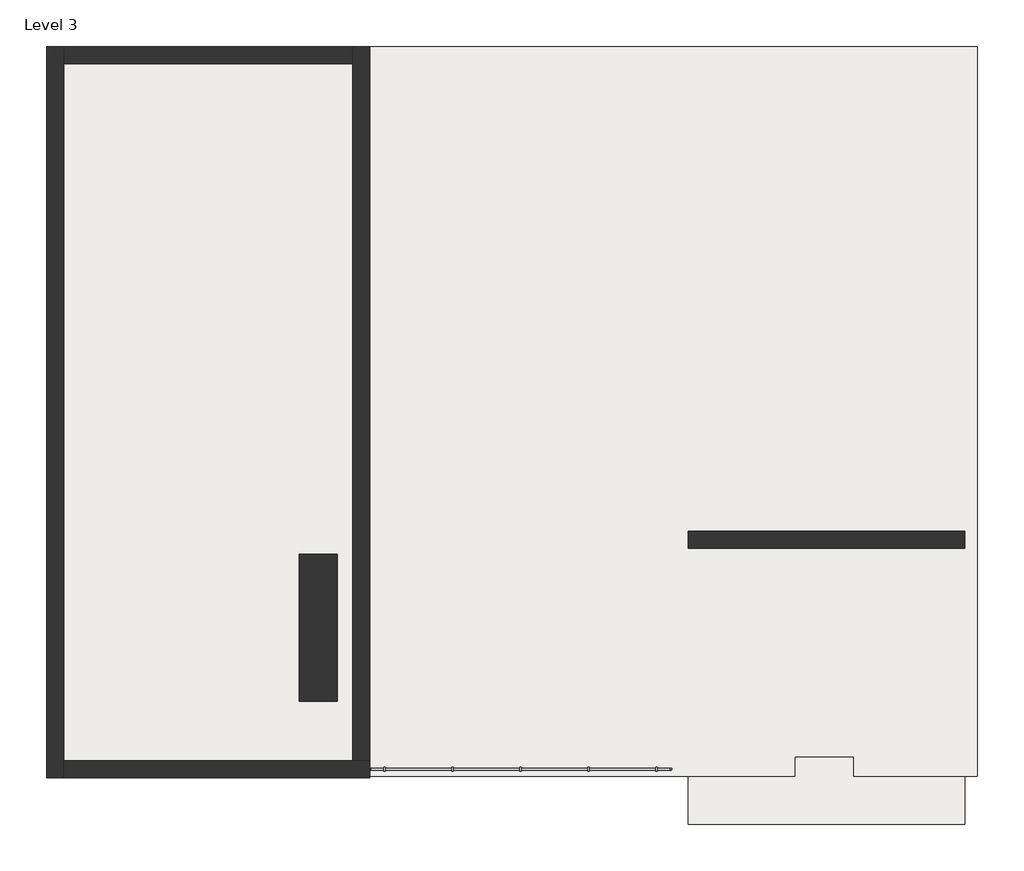
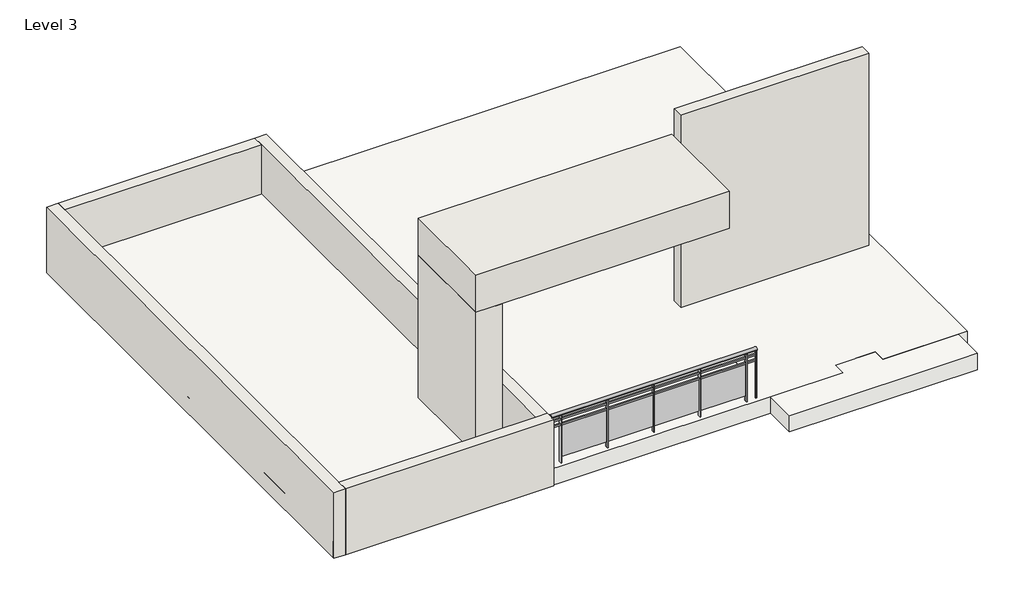
# One storey: 6 walls, 2 roofs, 1 railing.
"""IFC4 building model written with IfcOpenShell, lengths in millimetres."""

from ifc_helpers import new_model, si_unit, point, frame, origin, place, context, project, spatial, polyline, ellipse_curve, trimmed, outline, extrude, faceted_brep, transform, mapped, element, save
from ifc_brep_helpers import plane_surface, extruded_surface, advanced_brep
from components import walls_1_walls_1_cd62c845

model = new_model("IFC4")

# Units and contexts
model_context = context("Model", 3, world=origin())
ifc_project = project(units=[si_unit("LENGTHUNIT", "METRE", prefix="MILLI")], contexts=[model_context])

# Site, building, storey
site = spatial("IfcSite", under=ifc_project)
building = spatial("IfcBuilding", under=site)
storey = spatial("IfcBuildingStorey", under=building, Name="Level 3", Elevation=7315.2)

# Railing
placement = place(None, origin())
element("IfcRailing", 1, ObjectType="Glass Panel - Bottom Fill", at=placement, inside=storey, context=model_context, shape_type="SolidModel", body=[
    advanced_brep(
    [(-8888.211895, -256.3574077, 8534.4), (-8888.211895, -332.5574077, 8534.4), (-5281.411895, -256.3574077, 8534.4), (-5281.411895, -332.5574077, 8534.4)],
    [
        (0, 1, ellipse_curve(frame((-8888.211895, -294.4574077, 8534.4), z_axis=(-1.0, 0.0, 0.0), x_axis=(0.0, -1.0, 0.0)), 38.1, 28.575)),
        (1, 0, ellipse_curve(frame((-8888.211895, -294.4574077, 8534.4), z_axis=(-1.0, 0.0, 0.0), x_axis=(0.0, -1.0, 0.0)), 38.1, 28.575)),
        (2, 3, ellipse_curve(frame((-5281.411895, -294.4574077, 8534.4), z_axis=(1.0, 0.0, 0.0), x_axis=(0.0, -1.0, 0.0)), 38.1, 28.575)),
        (3, 2, ellipse_curve(frame((-5281.411895, -294.4574077, 8534.4), z_axis=(1.0, 0.0, 0.0), x_axis=(0.0, -1.0, 0.0)), 38.1, 28.575)),
        (0, 2),
        (3, 1),
    ],
    [
        plane_surface(frame((-8888.211895, -294.4574077, 8534.4), z_axis=(-1.0, 0.0, 0.0), x_axis=(0.0, 1.0, 0.0))),
        plane_surface(frame((-5281.411895, -294.4574077, 8534.4), z_axis=(1.0, 0.0, 0.0), x_axis=(0.0, 1.0, 0.0))),
        extruded_surface(trimmed(ellipse_curve(frame((-5281.411895, -294.4574077, 8534.4), z_axis=(-1.0, 0.0, 0.0), x_axis=(0.0, -1.0, 0.0)), 38.1, 28.575), [point((-5281.411895, -256.3574077, 8534.4))], [point((-5281.411895, -332.5574077, 8534.4))], True, "CARTESIAN"), (-3606.8, 0.0, 0.0), 3606.8),
        extruded_surface(trimmed(ellipse_curve(frame((-5281.411895, -294.4574077, 8534.4), z_axis=(-1.0, 0.0, 0.0), x_axis=(0.0, -1.0, 0.0)), 38.1, 28.575), [point((-5281.411895, -332.5574077, 8534.4))], [point((-5281.411895, -256.3574077, 8534.4))], True, "CARTESIAN"), (-3606.8, 0.0, 0.0), 3606.8),
    ],
    [
        (0, [[1, 2]]),
        (1, [[3, 4]]),
        (2, [[-1, 5, -4, 6]]),
        (3, [[-2, -6, -3, -5]]),
    ],
),
    extrude(outline(polyline([(-8888.211895, -307.1574077), (-8888.211895, -281.7574077), (-5281.411895, -281.7574077), (-5281.411895, -307.1574077), (-8888.211895, -307.1574077)])), frame((0.0, 0.0, 8420.1), z_axis=(0.0, 0.0, 1.0), x_axis=(1.0, 0.0, 0.0)), (0.0, 0.0, 1.0), 25.4),
    extrude(outline(polyline([(-8888.211895, -307.1574077), (-8888.211895, -281.7574077), (-5281.411895, -281.7574077), (-5281.411895, -307.1574077), (-8888.211895, -307.1574077)])), frame((0.0, 0.0, 8318.5), z_axis=(0.0, 0.0, 1.0), x_axis=(1.0, 0.0, 0.0)), (0.0, 0.0, 1.0), 25.4),
    extrude(outline(polyline([(-5465.561895, -319.8574077), (-5465.561895, -269.0574077), (-5452.861895, -269.0574077), (-5452.861895, -319.8574077), (-5465.561895, -319.8574077)])), frame((0.0, 0.0, 7620.0), z_axis=(0.0, 0.0, 1.0), x_axis=(1.0, 0.0, 0.0)), (0.0, 0.0, 1.0), 885.6788223),
    extrude(outline(polyline([(-6272.011895, -287.9222507), (-5459.211895, -287.9222507), (-5459.211895, -294.2722507), (-6272.011895, -294.2722507), (-6272.011895, -287.9222507)])), frame((0.0, 0.0, 7721.6), z_axis=(0.0, 0.0, 1.0), x_axis=(1.0, 0.0, 0.0)), (0.0, 0.0, 1.0), 596.9),
    extrude(outline(polyline([(-6278.361895, -319.8574077), (-6278.361895, -269.0574077), (-6265.661895, -269.0574077), (-6265.661895, -319.8574077), (-6278.361895, -319.8574077)])), frame((0.0, 0.0, 7620.0), z_axis=(0.0, 0.0, 1.0), x_axis=(1.0, 0.0, 0.0)), (0.0, 0.0, 1.0), 885.6788223),
    extrude(outline(polyline([(-7084.811895, -287.9222507), (-6272.011895, -287.9222507), (-6272.011895, -294.2722507), (-7084.811895, -294.2722507), (-7084.811895, -287.9222507)])), frame((0.0, 0.0, 7721.6), z_axis=(0.0, 0.0, 1.0), x_axis=(1.0, 0.0, 0.0)), (0.0, 0.0, 1.0), 596.9),
    extrude(outline(polyline([(-7091.161895, -319.8574077), (-7091.161895, -269.0574077), (-7078.461895, -269.0574077), (-7078.461895, -319.8574077), (-7091.161895, -319.8574077)])), frame((0.0, 0.0, 7620.0), z_axis=(0.0, 0.0, 1.0), x_axis=(1.0, 0.0, 0.0)), (0.0, 0.0, 1.0), 885.6788223),
    extrude(outline(polyline([(-7897.611895, -287.9222507), (-7084.811895, -287.9222507), (-7084.811895, -294.2722507), (-7897.611895, -294.2722507), (-7897.611895, -287.9222507)])), frame((0.0, 0.0, 7721.6), z_axis=(0.0, 0.0, 1.0), x_axis=(1.0, 0.0, 0.0)), (0.0, 0.0, 1.0), 596.9),
    extrude(outline(polyline([(-7903.961895, -319.8574077), (-7903.961895, -269.0574077), (-7891.261895, -269.0574077), (-7891.261895, -319.8574077), (-7903.961895, -319.8574077)])), frame((0.0, 0.0, 7620.0), z_axis=(0.0, 0.0, 1.0), x_axis=(1.0, 0.0, 0.0)), (0.0, 0.0, 1.0), 885.6788223),
    extrude(outline(polyline([(-8710.411895, -287.9222507), (-7897.611895, -287.9222507), (-7897.611895, -294.2722507), (-8710.411895, -294.2722507), (-8710.411895, -287.9222507)])), frame((0.0, 0.0, 7721.6), z_axis=(0.0, 0.0, 1.0), x_axis=(1.0, 0.0, 0.0)), (0.0, 0.0, 1.0), 596.9),
    extrude(outline(polyline([(-8716.761895, -319.8574077), (-8716.761895, -269.0574077), (-8704.061895, -269.0574077), (-8704.061895, -319.8574077), (-8716.761895, -319.8574077)])), frame((0.0, 0.0, 7620.0), z_axis=(0.0, 0.0, 1.0), x_axis=(1.0, 0.0, 0.0)), (0.0, 0.0, 1.0), 885.6788223),
    extrude(outline(polyline([(-5294.111895, -303.9824077), (-5294.111895, -284.9324077), (-5275.061895, -284.9324077), (-5275.061895, -303.9824077), (-5294.111895, -303.9824077)])), frame((0.0, 0.0, 7620.0), z_axis=(0.0, 0.0, 1.0), x_axis=(1.0, 0.0, 0.0)), (0.0, 0.0, 1.0), 885.6788223),
    extrude(outline(polyline([(-8894.561895, -303.9824077), (-8894.561895, -284.9324077), (-8875.511895, -284.9324077), (-8875.511895, -303.9824077), (-8894.561895, -303.9824077)])), frame((0.0, 0.0, 7620.0), z_axis=(0.0, 0.0, 1.0), x_axis=(1.0, 0.0, 0.0)), (0.0, 0.0, 1.0), 885.6788223),
])

# Roofs
element("IfcRoof", 2, ObjectType="Generic - 12\"", at=placement, inside=storey, context=model_context, shape_type="SweptSolid", body=[
    extrude(outline(polyline([(-5078.211895, 2347.1425923), (-1776.211895, 2347.1425923), (-1776.211895, -954.8574077), (-5078.211895, -954.8574077), (-5078.211895, 2347.1425923)])), frame((0.0, 0.0, 7315.2), z_axis=(0.0, 0.0, 1.0), x_axis=(1.0, 0.0, 0.0)), (0.0, 0.0, 1.0), 304.8),
])
element("IfcRoof", 3, ObjectType="Generic - 12\"", at=placement, inside=storey, context=model_context, shape_type="SweptSolid", body=[
    extrude(outline(polyline([(-12749.011895, 8341.5425923), (-1623.5722278, 8341.5425923), (-1623.5722278, -377.0074077), (-3103.4757185, -377.0074077), (-3103.4757185, -148.6618819), (-3805.5739054, -148.6618819), (-3805.5739054, -377.2618819), (-12749.011895, -377.2618819), (-12749.011895, 8341.5425923)])), frame((0.0, 0.0, 7315.2), z_axis=(0.0, 0.0, 1.0), x_axis=(1.0, 0.0, 0.0)), (0.0, 0.0, 1.0), 304.8),
])

# Walls
element("IfcWall", 4, ObjectType="Generic - 8\"", at=placement, inside=storey, context=model_context, shape_type="Brep", body=[
    faceted_brep([(-12749.011895, 8341.5425923, 7315.2), (-12749.011895, -396.0574077, 7315.2), (-12749.011895, -396.0574077, 8534.4), (-12749.011895, 8341.5425923, 8534.4), (-12545.811895, 8341.5425923, 7315.2), (-12545.811895, 8341.5425923, 8534.4), (-12545.811895, 8138.3425923, 8534.4), (-12545.811895, -192.8574077, 8534.4), (-12545.811895, -396.0574077, 8534.4), (-12545.811895, -396.0574077, 7315.2), (-12545.811895, -192.8574077, 7315.2), (-12545.811895, 8138.3425923, 7315.2)], [[[0, 1, 2, 3]], [[4, 5, 6, 7, 8, 9, 10, 11]], [[1, 0, 4, 11, 10, 9]], [[3, 2, 8, 7, 6, 5]], [[2, 1, 9, 8]], [[0, 3, 5, 4]]]),
])
element("IfcWall", 5, ObjectType="Generic - 8\"", at=placement, inside=storey, context=model_context, shape_type="Brep", body=[
    faceted_brep([(-12545.811895, -396.0574077, 7315.2), (-8888.211895, -396.0574077, 7315.2), (-8888.211895, -396.0574077, 8534.4), (-12545.811895, -396.0574077, 8534.4), (-12545.811895, -192.8574077, 7315.2), (-12545.811895, -192.8574077, 8534.4), (-9091.411895, -192.8574077, 8534.4), (-8888.211895, -192.8574077, 8534.4), (-8888.211895, -192.8574077, 7315.2), (-9091.411895, -192.8574077, 7315.2)], [[[0, 1, 2, 3]], [[4, 5, 6, 7, 8, 9]], [[1, 0, 4, 9, 8]], [[3, 2, 7, 6, 5]], [[0, 3, 5, 4]], [[2, 1, 8, 7]]]),
])
element("IfcWall", 6, ObjectType="Generic - 8\"", at=placement, inside=storey, context=model_context, shape_type="Brep", body=[
    faceted_brep([(-8888.211895, -192.8574077, 7315.2), (-8888.211895, 8341.5425923, 7315.2), (-8888.211895, 8341.5425923, 8534.4), (-8888.211895, -192.8574077, 8534.4), (-9091.411895, -192.8574077, 7315.2), (-9091.411895, -192.8574077, 8534.4), (-9091.411895, 8138.3425923, 8534.4), (-9091.411895, 8341.5425923, 8534.4), (-9091.411895, 8341.5425923, 7315.2), (-9091.411895, 8138.3425923, 7315.2)], [[[0, 1, 2, 3]], [[4, 5, 6, 7, 8, 9]], [[1, 0, 4, 9, 8]], [[3, 2, 7, 6, 5]], [[0, 3, 5, 4]], [[2, 1, 8, 7]]]),
])
element("IfcWall", 7, ObjectType="Generic - 8\"", at=placement, inside=storey, context=model_context, shape_type="SweptSolid", body=[
    extrude(outline(polyline([(-12545.811895, 8341.5425923), (-9091.411895, 8341.5425923), (-9091.411895, 8138.3425923), (-12545.811895, 8138.3425923), (-12545.811895, 8341.5425923)])), frame((0.0, 0.0, 7315.2), z_axis=(0.0, 0.0, 1.0), x_axis=(1.0, 0.0, 0.0)), (0.0, 0.0, 1.0), 1219.2),
])
element("IfcWall", 8, ObjectType="Generic - 8\"", at=placement, inside=storey, context=model_context, shape_type="Brep", body=[
    faceted_brep([(-5078.211895, 2347.1425923, 7315.2), (-1776.211895, 2347.1425923, 7315.2), (-1776.211895, 2347.1425923, 11185.4130687), (-5078.211895, 2347.1425923, 11185.4130687), (-5078.211895, 2550.3425923, 7315.2), (-5078.211895, 2550.3425923, 11185.4130687), (-1776.211895, 2550.3425923, 11185.4130687), (-1776.211895, 2550.3425923, 7315.2), (-1776.211895, 2448.7425923, 7315.2)], [[[0, 1, 2, 3]], [[4, 5, 6, 7]], [[1, 0, 4, 7, 8]], [[3, 2, 6, 5]], [[2, 1, 8, 7, 6]], [[0, 3, 5, 4]]]),
])
walls_1_walls_1_shape = walls_1_walls_1_cd62c845(model_context)
element("IfcWall", 9, ObjectType="Walls 1 : Walls 1", at=placement, inside=storey, context=model_context, shape_type="MappedRepresentation", body=[
    mapped(walls_1_walls_1_shape, transform((0.0, 0.0, 0.0), x_axis=(1.0, 0.0, 0.0), y_axis=(0.0, 1.0, 0.0), z_axis=(0.0, 0.0, 1.0))),
])

save(model, "model.ifc")

# Revit data of these elements
# Type "Glass Panel - Bottom Fill"
#   Assembly Code = "C2010400"
#   built-in parameter 1008612 = 0.0416667 (stored number, unit not read)
#   built-in parameter 1008611 = 0.0416667 (stored number, unit not read)
#   built-in parameter 1008609 = 0.333333 (stored number, unit not read)
#   built-in parameter 1008604 = 0.166667 (stored number, unit not read)
#   built-in parameter 1008603 = 0.166667 (stored number, unit not read)
#   Railing Height = 3' - 0"
#   built-in parameter 1008630 = 2
#   built-in parameter 1008610 = 2
#   built-in parameter 1008618 = Baluster - Square : 3/4"
# Type "Generic - 12\""
#   Assembly Code = "B1020"
#   Layers, outside or top first: 1' - 0" no material (function 1)
# Type "Generic - 8\""
#   Assembly Code = "B2010"
#   Layers, outside or top first: 0' - 8" no material (function 1)
# Element 1 (IfcRailing, "Glass Panel - Bottom Fill")
#   built-in parameter 1008621 = 1 (stored number, unit not read)
#   Phase Created = New Construction
#   Materials on its faces: "Glass"
# Elements 2, 3 (IfcRoof, "Generic - 12\"")
#   built-in parameter 1001705 = 25 (stored number, unit not read)
#   built-in parameter 1001710 = 33615
#   Phase Created = New Construction
#   Materials on its faces: "Default Roof"
# Elements 4, 5, 6, 7 (IfcWall, "Generic - 8\"")
#   Top Offset = 0' - 0"
#   Base Offset = 0' - 0"
#   Unconnected Height = 4' - 0"
#   wall height = 4' - 0"
#   Phase Created = New Construction
#   Base Constraint = Level 3
#   Materials on its faces: "Default Wall"
# Element 8 (IfcWall, "Generic - 8\"")
#   Top Offset = 0' - 0"
#   Base Offset = 0' - 0"
#   Unconnected Height = 12' - 8.37059"
#   wall height = 12' - 8.37059"
#   Phase Created = New Construction
#   Base Constraint = Level 3
#   Materials on its faces: "Default Wall"
# Element 9 (IfcWall, "Walls 1 : Walls 1")
#   Phase Created = New Construction
#   Materials on its faces: "Default Wall"
# Materials
#   "Glass": class "Glass", colour RGB 0 128 192, transparency 0.75, Description = "Soda Lime Glass", Cost = 0
#   "Default Roof": colour RGB 88 101 114, transparency 0
#   "Default Wall": colour RGB 128 128 128, transparency 0
